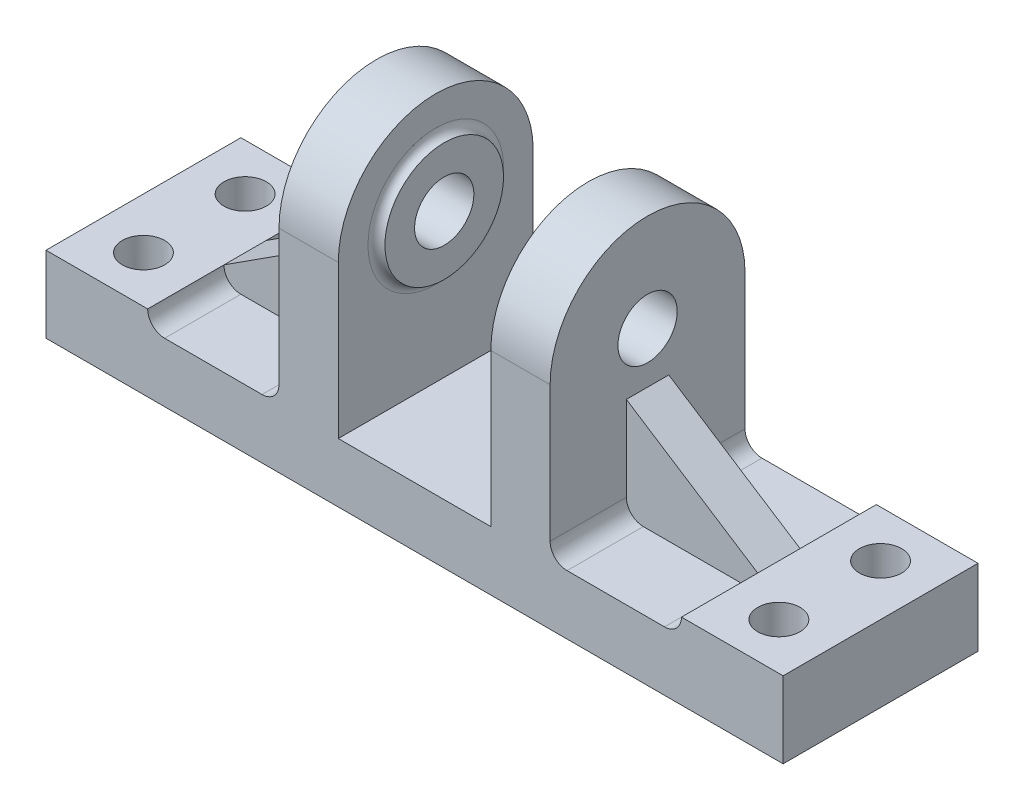
ISO-10303-21;
HEADER;
FILE_DESCRIPTION(('STEP AP214'),'2;1');
FILE_NAME('part.step','',(''),(''),'','','');
FILE_SCHEMA(('AUTOMOTIVE_DESIGN { 1 0 10303 214 1 1 1 1 }'));
ENDSEC;
DATA;
#1=APPLICATION_CONTEXT('core data for automotive mechanical design processes');
#2=APPLICATION_PROTOCOL_DEFINITION('international standard','automotive_design',2000,#1);
#3=PRODUCT_CONTEXT('',#1,'mechanical');
#4=PRODUCT('Part','Part','',(#3));
#5=PRODUCT_RELATED_PRODUCT_CATEGORY('part','',(#4));
#6=PRODUCT_DEFINITION_FORMATION('','',#4);
#7=PRODUCT_DEFINITION_CONTEXT('part definition',#1,'design');
#8=PRODUCT_DEFINITION('design','',#6,#7);
#9=PRODUCT_DEFINITION_SHAPE('','',#8);
#10=(LENGTH_UNIT() NAMED_UNIT(*) SI_UNIT(.MILLI.,.METRE.));
#11=(NAMED_UNIT(*) PLANE_ANGLE_UNIT() SI_UNIT($,.RADIAN.));
#12=(NAMED_UNIT(*) SI_UNIT($,.STERADIAN.) SOLID_ANGLE_UNIT());
#13=UNCERTAINTY_MEASURE_WITH_UNIT(LENGTH_MEASURE(1.E-05),#10,'distance_accuracy_value','');
#14=(GEOMETRIC_REPRESENTATION_CONTEXT(3) GLOBAL_UNCERTAINTY_ASSIGNED_CONTEXT((#13)) GLOBAL_UNIT_ASSIGNED_CONTEXT((#10,
#11,#12)) REPRESENTATION_CONTEXT('',''));
#15=CARTESIAN_POINT('',(0.,0.,0.));
#16=DIRECTION('',(0.,0.,1.));
#17=DIRECTION('',(1.,0.,0.));
#18=AXIS2_PLACEMENT_3D('',#15,#16,#17);
#19=CARTESIAN_POINT('',(63.,5.00000000000001,23.));
#20=DIRECTION('',(0.,-1.,0.));
#21=DIRECTION('',(1.,0.,0.));
#22=AXIS2_PLACEMENT_3D('',#19,#20,#21);
#23=PLANE('',#22);
#24=DIRECTION('',(-1.,0.,0.));
#25=VECTOR('',#24,1.);
#26=CARTESIAN_POINT('',(63.,5.00000000000001,-5.));
#27=LINE('',#26,#25);
#28=CARTESIAN_POINT('',(-36.,5.,-5.));
#29=VERTEX_POINT('',#28);
#30=CARTESIAN_POINT('',(-59.,5.,-5.));
#31=VERTEX_POINT('',#30);
#32=EDGE_CURVE('E245',#29,#31,#27,.T.);
#33=ORIENTED_EDGE('',*,*,#32,.F.);
#34=DIRECTION('',(0.,0.,-1.));
#35=VECTOR('',#34,1.);
#36=CARTESIAN_POINT('',(-36.,5.,23.));
#37=LINE('',#36,#35);
#38=CARTESIAN_POINT('',(-36.,5.,-23.));
#39=VERTEX_POINT('',#38);
#40=EDGE_CURVE('E227',#29,#39,#37,.T.);
#41=ORIENTED_EDGE('',*,*,#40,.T.);
#42=DIRECTION('',(-1.,0.,0.));
#43=VECTOR('',#42,1.);
#44=CARTESIAN_POINT('',(63.,5.00000000000001,-23.));
#45=LINE('',#44,#43);
#46=CARTESIAN_POINT('',(-59.,5.,-23.));
#47=VERTEX_POINT('',#46);
#48=EDGE_CURVE('E328',#39,#47,#45,.T.);
#49=ORIENTED_EDGE('',*,*,#48,.T.);
#50=DIRECTION('',(0.,0.,-1.));
#51=VECTOR('',#50,1.);
#52=CARTESIAN_POINT('',(-59.,5.,23.));
#53=LINE('',#52,#51);
#54=EDGE_CURVE('E242',#47,#31,#53,.F.);
#55=ORIENTED_EDGE('',*,*,#54,.T.);
#56=EDGE_LOOP('',(#33,#41,#49,#55));
#57=FACE_BOUND('',#56,.T.);
#58=ADVANCED_FACE('F41',(#57),#23,.F.);
#59=CARTESIAN_POINT('',(-59.,9.,23.));
#60=DIRECTION('',(0.,0.,1.));
#61=DIRECTION('',(1.,0.,0.));
#62=AXIS2_PLACEMENT_3D('',#59,#60,#61);
#63=CYLINDRICAL_SURFACE('',#62,4.);
#64=CARTESIAN_POINT('',(-59.,9.,-5.));
#65=DIRECTION('',(0.,0.,1.));
#66=DIRECTION('',(1.,0.,0.));
#67=AXIS2_PLACEMENT_3D('',#64,#65,#66);
#68=CIRCLE('',#67,4.);
#69=CARTESIAN_POINT('',(-63.,8.99999999999999,-5.));
#70=VERTEX_POINT('',#69);
#71=EDGE_CURVE('E250',#31,#70,#68,.F.);
#72=ORIENTED_EDGE('',*,*,#71,.F.);
#73=ORIENTED_EDGE('',*,*,#54,.F.);
#74=CARTESIAN_POINT('',(-59.,9.,-23.));
#75=DIRECTION('',(0.,0.,1.));
#76=DIRECTION('',(1.,0.,0.));
#77=AXIS2_PLACEMENT_3D('',#74,#75,#76);
#78=CIRCLE('',#77,4.);
#79=CARTESIAN_POINT('',(-63.,8.99999999999999,-23.));
#80=VERTEX_POINT('',#79);
#81=EDGE_CURVE('E286',#80,#47,#78,.T.);
#82=ORIENTED_EDGE('',*,*,#81,.F.);
#83=DIRECTION('',(0.,0.,-1.));
#84=VECTOR('',#83,1.);
#85=CARTESIAN_POINT('',(-63.,8.99999999999999,23.));
#86=LINE('',#85,#84);
#87=EDGE_CURVE('E57',#70,#80,#86,.T.);
#88=ORIENTED_EDGE('',*,*,#87,.F.);
#89=EDGE_LOOP('',(#72,#73,#82,#88));
#90=FACE_BOUND('',#89,.T.);
#91=ADVANCED_FACE('F595',(#90),#63,.F.);
#92=CARTESIAN_POINT('',(-36.,9.,23.));
#93=DIRECTION('',(0.,0.,-1.));
#94=DIRECTION('',(-1.,0.,0.));
#95=AXIS2_PLACEMENT_3D('',#92,#93,#94);
#96=CYLINDRICAL_SURFACE('',#95,4.);
#97=CARTESIAN_POINT('',(-36.,9.,-5.));
#98=DIRECTION('',(0.,0.,1.));
#99=DIRECTION('',(1.,0.,0.));
#100=AXIS2_PLACEMENT_3D('',#97,#98,#99);
#101=CIRCLE('',#100,4.);
#102=CARTESIAN_POINT('',(-32.,9.,-5.));
#103=VERTEX_POINT('',#102);
#104=EDGE_CURVE('E235',#103,#29,#101,.F.);
#105=ORIENTED_EDGE('',*,*,#104,.F.);
#106=DIRECTION('',(0.,0.,-1.));
#107=VECTOR('',#106,1.);
#108=CARTESIAN_POINT('',(-32.,9.,0.));
#109=LINE('',#108,#107);
#110=CARTESIAN_POINT('',(-32.,9.,-23.));
#111=VERTEX_POINT('',#110);
#112=EDGE_CURVE('E259',#111,#103,#109,.F.);
#113=ORIENTED_EDGE('',*,*,#112,.F.);
#114=CARTESIAN_POINT('',(-36.,9.,-23.));
#115=DIRECTION('',(0.,0.,1.));
#116=DIRECTION('',(1.,0.,0.));
#117=AXIS2_PLACEMENT_3D('',#114,#115,#116);
#118=CIRCLE('',#117,4.);
#119=EDGE_CURVE('E234',#39,#111,#118,.T.);
#120=ORIENTED_EDGE('',*,*,#119,.F.);
#121=ORIENTED_EDGE('',*,*,#40,.F.);
#122=EDGE_LOOP('',(#105,#113,#120,#121));
#123=FACE_BOUND('',#122,.T.);
#124=ADVANCED_FACE('F230',(#123),#96,.F.);
#125=CARTESIAN_POINT('',(-18.,0.,0.));
#126=DIRECTION('',(-1.,0.,0.));
#127=DIRECTION('',(0.,0.,-1.));
#128=AXIS2_PLACEMENT_3D('',#125,#126,#127);
#129=PLANE('',#128);
#130=CARTESIAN_POINT('',(-18.,41.,0.));
#131=DIRECTION('',(-1.,0.,0.));
#132=DIRECTION('',(0.,0.,1.));
#133=AXIS2_PLACEMENT_3D('',#130,#131,#132);
#134=CIRCLE('',#133,16.);
#135=CARTESIAN_POINT('',(-18.,41.,16.));
#136=VERTEX_POINT('',#135);
#137=EDGE_CURVE('E238',#136,#136,#134,.T.);
#138=ORIENTED_EDGE('',*,*,#137,.T.);
#139=EDGE_LOOP('',(#138));
#140=FACE_BOUND('',#139,.T.);
#141=DIRECTION('',(0.,0.,-1.));
#142=VECTOR('',#141,1.);
#143=CARTESIAN_POINT('',(-18.,5.00000000000002,0.));
#144=LINE('',#143,#142);
#145=CARTESIAN_POINT('',(-18.,5.,23.));
#146=VERTEX_POINT('',#145);
#147=CARTESIAN_POINT('',(-18.,5.,-23.));
#148=VERTEX_POINT('',#147);
#149=EDGE_CURVE('E453',#146,#148,#144,.T.);
#150=ORIENTED_EDGE('',*,*,#149,.T.);
#151=DIRECTION('',(0.,-1.,0.));
#152=VECTOR('',#151,1.);
#153=CARTESIAN_POINT('',(-18.,0.,-23.));
#154=LINE('',#153,#152);
#155=CARTESIAN_POINT('',(-18.,41.,-23.));
#156=VERTEX_POINT('',#155);
#157=EDGE_CURVE('E459',#156,#148,#154,.T.);
#158=ORIENTED_EDGE('',*,*,#157,.F.);
#159=CARTESIAN_POINT('',(-18.,41.,0.));
#160=DIRECTION('',(1.,0.,0.));
#161=DIRECTION('',(0.,0.,-1.));
#162=AXIS2_PLACEMENT_3D('',#159,#160,#161);
#163=CIRCLE('',#162,23.);
#164=CARTESIAN_POINT('',(-18.,41.,23.));
#165=VERTEX_POINT('',#164);
#166=EDGE_CURVE('E445',#165,#156,#163,.F.);
#167=ORIENTED_EDGE('',*,*,#166,.F.);
#168=DIRECTION('',(0.,-1.,0.));
#169=VECTOR('',#168,1.);
#170=CARTESIAN_POINT('',(-18.,0.,23.));
#171=LINE('',#170,#169);
#172=EDGE_CURVE('E440',#165,#146,#171,.T.);
#173=ORIENTED_EDGE('',*,*,#172,.T.);
#174=EDGE_LOOP('',(#150,#158,#167,#173));
#175=FACE_BOUND('',#174,.T.);
#176=ADVANCED_FACE('F515',(#140,#175),#129,.F.);
#177=DIRECTION('',(0.,0.,-1.));
#178=VECTOR('',#177,1.);
#179=CARTESIAN_POINT('',(18.,5.00000000000002,0.));
#180=LINE('',#179,#178);
#181=CARTESIAN_POINT('',(18.,5.,23.));
#182=VERTEX_POINT('',#181);
#183=CARTESIAN_POINT('',(18.,5.00000000000002,-23.));
#184=VERTEX_POINT('',#183);
#185=EDGE_CURVE('E399',#182,#184,#180,.T.);
#186=ORIENTED_EDGE('',*,*,#185,.T.);
#187=EDGE_CURVE('E323',#184,#148,#45,.T.);
#188=ORIENTED_EDGE('',*,*,#187,.T.);
#189=ORIENTED_EDGE('',*,*,#149,.F.);
#190=DIRECTION('',(-1.,0.,0.));
#191=VECTOR('',#190,1.);
#192=CARTESIAN_POINT('',(63.,5.00000000000001,23.));
#193=LINE('',#192,#191);
#194=EDGE_CURVE('E341',#182,#146,#193,.T.);
#195=ORIENTED_EDGE('',*,*,#194,.F.);
#196=EDGE_LOOP('',(#186,#188,#189,#195));
#197=FACE_BOUND('',#196,.T.);
#198=ADVANCED_FACE('F525',(#197),#23,.F.);
#199=DIRECTION('',(-1.,0.,0.));
#200=VECTOR('',#199,1.);
#201=CARTESIAN_POINT('',(63.,5.00000000000001,-5.));
#202=LINE('',#201,#200);
#203=CARTESIAN_POINT('',(59.,5.00000000000001,-5.));
#204=VERTEX_POINT('',#203);
#205=CARTESIAN_POINT('',(36.,5.00000000000001,-5.));
#206=VERTEX_POINT('',#205);
#207=EDGE_CURVE('E422',#204,#206,#202,.T.);
#208=ORIENTED_EDGE('',*,*,#207,.F.);
#209=DIRECTION('',(0.,0.,-1.));
#210=VECTOR('',#209,1.);
#211=CARTESIAN_POINT('',(59.,5.00000000000001,-23.));
#212=LINE('',#211,#210);
#213=CARTESIAN_POINT('',(59.,5.00000000000001,-23.));
#214=VERTEX_POINT('',#213);
#215=EDGE_CURVE('E297',#204,#214,#212,.T.);
#216=ORIENTED_EDGE('',*,*,#215,.T.);
#217=CARTESIAN_POINT('',(36.,5.00000000000001,-23.));
#218=VERTEX_POINT('',#217);
#219=EDGE_CURVE('E325',#214,#218,#45,.T.);
#220=ORIENTED_EDGE('',*,*,#219,.T.);
#221=DIRECTION('',(0.,0.,-1.));
#222=VECTOR('',#221,1.);
#223=CARTESIAN_POINT('',(36.,5.00000000000001,23.));
#224=LINE('',#223,#222);
#225=EDGE_CURVE('E277',#218,#206,#224,.F.);
#226=ORIENTED_EDGE('',*,*,#225,.T.);
#227=EDGE_LOOP('',(#208,#216,#220,#226));
#228=FACE_BOUND('',#227,.T.);
#229=ADVANCED_FACE('F542',(#228),#23,.F.);
#230=CARTESIAN_POINT('',(59.,9.00000000000001,23.));
#231=DIRECTION('',(0.,0.,1.));
#232=DIRECTION('',(1.,0.,0.));
#233=AXIS2_PLACEMENT_3D('',#230,#231,#232);
#234=CYLINDRICAL_SURFACE('',#233,4.);
#235=CARTESIAN_POINT('',(59.,9.00000000000001,-5.));
#236=DIRECTION('',(0.,0.,1.));
#237=DIRECTION('',(1.,0.,0.));
#238=AXIS2_PLACEMENT_3D('',#235,#236,#237);
#239=CIRCLE('',#238,4.);
#240=CARTESIAN_POINT('',(63.,9.00000000000001,-5.));
#241=VERTEX_POINT('',#240);
#242=EDGE_CURVE('E416',#241,#204,#239,.F.);
#243=ORIENTED_EDGE('',*,*,#242,.F.);
#244=DIRECTION('',(0.,0.,-1.));
#245=VECTOR('',#244,1.);
#246=CARTESIAN_POINT('',(63.,9.00000000000001,23.));
#247=LINE('',#246,#245);
#248=CARTESIAN_POINT('',(63.,9.00000000000001,-23.));
#249=VERTEX_POINT('',#248);
#250=EDGE_CURVE('E315',#241,#249,#247,.T.);
#251=ORIENTED_EDGE('',*,*,#250,.T.);
#252=CARTESIAN_POINT('',(59.,9.00000000000001,-23.));
#253=DIRECTION('',(0.,0.,1.));
#254=DIRECTION('',(1.,0.,0.));
#255=AXIS2_PLACEMENT_3D('',#252,#253,#254);
#256=CIRCLE('',#255,4.);
#257=EDGE_CURVE('E295',#214,#249,#256,.T.);
#258=ORIENTED_EDGE('',*,*,#257,.F.);
#259=ORIENTED_EDGE('',*,*,#215,.F.);
#260=EDGE_LOOP('',(#243,#251,#258,#259));
#261=FACE_BOUND('',#260,.T.);
#262=ADVANCED_FACE('F548',(#261),#234,.F.);
#263=CARTESIAN_POINT('',(36.,9.00000000000001,0.));
#264=DIRECTION('',(0.,0.,-1.));
#265=DIRECTION('',(-1.,0.,0.));
#266=AXIS2_PLACEMENT_3D('',#263,#264,#265);
#267=CYLINDRICAL_SURFACE('',#266,4.);
#268=CARTESIAN_POINT('',(36.,9.00000000000001,-5.));
#269=DIRECTION('',(0.,0.,1.));
#270=DIRECTION('',(1.,0.,0.));
#271=AXIS2_PLACEMENT_3D('',#268,#269,#270);
#272=CIRCLE('',#271,4.);
#273=CARTESIAN_POINT('',(32.,9.00000000000001,-5.));
#274=VERTEX_POINT('',#273);
#275=EDGE_CURVE('E266',#206,#274,#272,.F.);
#276=ORIENTED_EDGE('',*,*,#275,.F.);
#277=ORIENTED_EDGE('',*,*,#225,.F.);
#278=CARTESIAN_POINT('',(36.,9.00000000000001,-23.));
#279=DIRECTION('',(0.,0.,1.));
#280=DIRECTION('',(1.,0.,0.));
#281=AXIS2_PLACEMENT_3D('',#278,#279,#280);
#282=CIRCLE('',#281,4.);
#283=CARTESIAN_POINT('',(32.,9.00000000000001,-23.));
#284=VERTEX_POINT('',#283);
#285=EDGE_CURVE('E274',#284,#218,#282,.T.);
#286=ORIENTED_EDGE('',*,*,#285,.F.);
#287=DIRECTION('',(0.,0.,-1.));
#288=VECTOR('',#287,1.);
#289=CARTESIAN_POINT('',(32.,9.00000000000001,0.));
#290=LINE('',#289,#288);
#291=EDGE_CURVE('E282',#274,#284,#290,.T.);
#292=ORIENTED_EDGE('',*,*,#291,.F.);
#293=EDGE_LOOP('',(#276,#277,#286,#292));
#294=FACE_BOUND('',#293,.T.);
#295=ADVANCED_FACE('F543',(#294),#267,.F.);
#296=CARTESIAN_POINT('',(-36.,5.,23.));
#297=VERTEX_POINT('',#296);
#298=CARTESIAN_POINT('',(-36.,5.,5.));
#299=VERTEX_POINT('',#298);
#300=EDGE_CURVE('E240',#297,#299,#37,.T.);
#301=ORIENTED_EDGE('',*,*,#300,.T.);
#302=DIRECTION('',(-1.,0.,0.));
#303=VECTOR('',#302,1.);
#304=CARTESIAN_POINT('',(63.,5.00000000000001,5.));
#305=LINE('',#304,#303);
#306=CARTESIAN_POINT('',(-59.,5.,5.));
#307=VERTEX_POINT('',#306);
#308=EDGE_CURVE('E468',#299,#307,#305,.T.);
#309=ORIENTED_EDGE('',*,*,#308,.T.);
#310=CARTESIAN_POINT('',(-59.,5.,23.));
#311=VERTEX_POINT('',#310);
#312=EDGE_CURVE('E305',#307,#311,#53,.F.);
#313=ORIENTED_EDGE('',*,*,#312,.T.);
#314=EDGE_CURVE('E343',#297,#311,#193,.T.);
#315=ORIENTED_EDGE('',*,*,#314,.F.);
#316=EDGE_LOOP('',(#301,#309,#313,#315));
#317=FACE_BOUND('',#316,.T.);
#318=ADVANCED_FACE('F502',(#317),#23,.F.);
#319=CARTESIAN_POINT('',(-87.,-9.,23.));
#320=DIRECTION('',(1.,0.,0.));
#321=DIRECTION('',(0.,0.,-1.));
#322=AXIS2_PLACEMENT_3D('',#319,#320,#321);
#323=PLANE('',#322);
#324=DIRECTION('',(0.,-1.,0.));
#325=VECTOR('',#324,1.);
#326=CARTESIAN_POINT('',(-87.,-9.,-23.));
#327=LINE('',#326,#325);
#328=CARTESIAN_POINT('',(-87.,9.,-23.));
#329=VERTEX_POINT('',#328);
#330=CARTESIAN_POINT('',(-87.,-9.,-23.));
#331=VERTEX_POINT('',#330);
#332=EDGE_CURVE('E337',#329,#331,#327,.T.);
#333=ORIENTED_EDGE('',*,*,#332,.T.);
#334=DIRECTION('',(0.,0.,-1.));
#335=VECTOR('',#334,1.);
#336=CARTESIAN_POINT('',(-87.,-9.,23.));
#337=LINE('',#336,#335);
#338=CARTESIAN_POINT('',(-87.,-9.,23.));
#339=VERTEX_POINT('',#338);
#340=EDGE_CURVE('E303',#339,#331,#337,.T.);
#341=ORIENTED_EDGE('',*,*,#340,.F.);
#342=DIRECTION('',(0.,-1.,0.));
#343=VECTOR('',#342,1.);
#344=CARTESIAN_POINT('',(-87.,-9.,23.));
#345=LINE('',#344,#343);
#346=CARTESIAN_POINT('',(-87.,9.,23.));
#347=VERTEX_POINT('',#346);
#348=EDGE_CURVE('E322',#347,#339,#345,.T.);
#349=ORIENTED_EDGE('',*,*,#348,.F.);
#350=DIRECTION('',(0.,0.,-1.));
#351=VECTOR('',#350,1.);
#352=CARTESIAN_POINT('',(-87.,9.,23.));
#353=LINE('',#352,#351);
#354=EDGE_CURVE('E314',#347,#329,#353,.T.);
#355=ORIENTED_EDGE('',*,*,#354,.T.);
#356=EDGE_LOOP('',(#333,#341,#349,#355));
#357=FACE_BOUND('',#356,.T.);
#358=ADVANCED_FACE('F614',(#357),#323,.F.);
#359=CARTESIAN_POINT('',(87.,-8.99999999999998,23.));
#360=DIRECTION('',(0.,1.,0.));
#361=DIRECTION('',(-1.,0.,0.));
#362=AXIS2_PLACEMENT_3D('',#359,#360,#361);
#363=PLANE('',#362);
#364=CARTESIAN_POINT('',(75.,-8.99999999999998,12.));
#365=DIRECTION('',(0.,1.,0.));
#366=DIRECTION('',(-1.,0.,0.));
#367=AXIS2_PLACEMENT_3D('',#364,#365,#366);
#368=CIRCLE('',#367,5.);
#369=CARTESIAN_POINT('',(70.,-8.99999999999998,12.));
#370=VERTEX_POINT('',#369);
#371=EDGE_CURVE('E358',#370,#370,#368,.T.);
#372=ORIENTED_EDGE('',*,*,#371,.T.);
#373=EDGE_LOOP('',(#372));
#374=FACE_BOUND('',#373,.T.);
#375=CARTESIAN_POINT('',(-75.,-9.,12.));
#376=DIRECTION('',(0.,1.,0.));
#377=DIRECTION('',(-1.,0.,0.));
#378=AXIS2_PLACEMENT_3D('',#375,#376,#377);
#379=CIRCLE('',#378,5.);
#380=CARTESIAN_POINT('',(-80.,-9.,12.));
#381=VERTEX_POINT('',#380);
#382=EDGE_CURVE('E360',#381,#381,#379,.T.);
#383=ORIENTED_EDGE('',*,*,#382,.T.);
#384=EDGE_LOOP('',(#383));
#385=FACE_BOUND('',#384,.T.);
#386=ORIENTED_EDGE('',*,*,#340,.T.);
#387=DIRECTION('',(1.,0.,0.));
#388=VECTOR('',#387,1.);
#389=CARTESIAN_POINT('',(87.,-8.99999999999998,-23.));
#390=LINE('',#389,#388);
#391=CARTESIAN_POINT('',(87.,-8.99999999999998,-23.));
#392=VERTEX_POINT('',#391);
#393=EDGE_CURVE('E334',#331,#392,#390,.T.);
#394=ORIENTED_EDGE('',*,*,#393,.T.);
#395=DIRECTION('',(0.,0.,-1.));
#396=VECTOR('',#395,1.);
#397=CARTESIAN_POINT('',(87.,-8.99999999999998,23.));
#398=LINE('',#397,#396);
#399=CARTESIAN_POINT('',(87.,-8.99999999999998,23.));
#400=VERTEX_POINT('',#399);
#401=EDGE_CURVE('E304',#400,#392,#398,.T.);
#402=ORIENTED_EDGE('',*,*,#401,.F.);
#403=DIRECTION('',(1.,0.,0.));
#404=VECTOR('',#403,1.);
#405=CARTESIAN_POINT('',(87.,-8.99999999999998,23.));
#406=LINE('',#405,#404);
#407=EDGE_CURVE('E346',#339,#400,#406,.T.);
#408=ORIENTED_EDGE('',*,*,#407,.F.);
#409=EDGE_LOOP('',(#386,#394,#402,#408));
#410=FACE_BOUND('',#409,.T.);
#411=CARTESIAN_POINT('',(75.,-8.99999999999998,-12.));
#412=DIRECTION('',(0.,1.,0.));
#413=DIRECTION('',(-1.,0.,0.));
#414=AXIS2_PLACEMENT_3D('',#411,#412,#413);
#415=CIRCLE('',#414,5.);
#416=CARTESIAN_POINT('',(70.,-8.99999999999998,-12.));
#417=VERTEX_POINT('',#416);
#418=EDGE_CURVE('E339',#417,#417,#415,.T.);
#419=ORIENTED_EDGE('',*,*,#418,.T.);
#420=EDGE_LOOP('',(#419));
#421=FACE_BOUND('',#420,.T.);
#422=CARTESIAN_POINT('',(-75.,-9.,-12.));
#423=DIRECTION('',(0.,1.,0.));
#424=DIRECTION('',(-1.,0.,0.));
#425=AXIS2_PLACEMENT_3D('',#422,#423,#424);
#426=CIRCLE('',#425,5.);
#427=CARTESIAN_POINT('',(-80.,-9.,-12.));
#428=VERTEX_POINT('',#427);
#429=EDGE_CURVE('E365',#428,#428,#426,.T.);
#430=ORIENTED_EDGE('',*,*,#429,.T.);
#431=EDGE_LOOP('',(#430));
#432=FACE_BOUND('',#431,.T.);
#433=ADVANCED_FACE('F617',(#374,#385,#410,#421,#432),#363,.F.);
#434=CARTESIAN_POINT('',(87.,-8.99999999999998,23.));
#435=DIRECTION('',(-1.,0.,0.));
#436=DIRECTION('',(0.,0.,1.));
#437=AXIS2_PLACEMENT_3D('',#434,#435,#436);
#438=PLANE('',#437);
#439=ORIENTED_EDGE('',*,*,#401,.T.);
#440=DIRECTION('',(0.,1.,0.));
#441=VECTOR('',#440,1.);
#442=CARTESIAN_POINT('',(87.,-8.99999999999998,-23.));
#443=LINE('',#442,#441);
#444=CARTESIAN_POINT('',(87.,9.00000000000002,-23.));
#445=VERTEX_POINT('',#444);
#446=EDGE_CURVE('E326',#392,#445,#443,.T.);
#447=ORIENTED_EDGE('',*,*,#446,.T.);
#448=DIRECTION('',(0.,0.,-1.));
#449=VECTOR('',#448,1.);
#450=CARTESIAN_POINT('',(87.,9.00000000000002,23.));
#451=LINE('',#450,#449);
#452=CARTESIAN_POINT('',(87.,9.00000000000002,23.));
#453=VERTEX_POINT('',#452);
#454=EDGE_CURVE('E310',#453,#445,#451,.T.);
#455=ORIENTED_EDGE('',*,*,#454,.F.);
#456=DIRECTION('',(0.,1.,0.));
#457=VECTOR('',#456,1.);
#458=CARTESIAN_POINT('',(87.,-8.99999999999998,23.));
#459=LINE('',#458,#457);
#460=EDGE_CURVE('E347',#400,#453,#459,.T.);
#461=ORIENTED_EDGE('',*,*,#460,.F.);
#462=EDGE_LOOP('',(#439,#447,#455,#461));
#463=FACE_BOUND('',#462,.T.);
#464=ADVANCED_FACE('F606',(#463),#438,.F.);
#465=CARTESIAN_POINT('',(87.,9.00000000000002,23.));
#466=DIRECTION('',(0.,-1.,0.));
#467=DIRECTION('',(1.,0.,0.));
#468=AXIS2_PLACEMENT_3D('',#465,#466,#467);
#469=PLANE('',#468);
#470=CARTESIAN_POINT('',(75.,8.99999999999998,12.));
#471=DIRECTION('',(0.,1.,0.));
#472=DIRECTION('',(-1.,0.,0.));
#473=AXIS2_PLACEMENT_3D('',#470,#471,#472);
#474=CIRCLE('',#473,5.);
#475=CARTESIAN_POINT('',(70.,8.99999999999998,12.));
#476=VERTEX_POINT('',#475);
#477=EDGE_CURVE('E375',#476,#476,#474,.T.);
#478=ORIENTED_EDGE('',*,*,#477,.F.);
#479=EDGE_LOOP('',(#478));
#480=FACE_BOUND('',#479,.T.);
#481=ORIENTED_EDGE('',*,*,#454,.T.);
#482=DIRECTION('',(-1.,0.,0.));
#483=VECTOR('',#482,1.);
#484=CARTESIAN_POINT('',(87.,9.00000000000002,-23.));
#485=LINE('',#484,#483);
#486=EDGE_CURVE('E329',#445,#249,#485,.T.);
#487=ORIENTED_EDGE('',*,*,#486,.T.);
#488=ORIENTED_EDGE('',*,*,#250,.F.);
#489=DIRECTION('',(0.,0.,1.));
#490=VECTOR('',#489,1.);
#491=CARTESIAN_POINT('',(63.,9.00000000000001,23.));
#492=LINE('',#491,#490);
#493=CARTESIAN_POINT('',(63.,9.00000000000001,5.));
#494=VERTEX_POINT('',#493);
#495=EDGE_CURVE('E408',#241,#494,#492,.T.);
#496=ORIENTED_EDGE('',*,*,#495,.T.);
#497=CARTESIAN_POINT('',(63.,9.00000000000001,23.));
#498=VERTEX_POINT('',#497);
#499=EDGE_CURVE('E307',#498,#494,#247,.T.);
#500=ORIENTED_EDGE('',*,*,#499,.F.);
#501=DIRECTION('',(-1.,0.,0.));
#502=VECTOR('',#501,1.);
#503=CARTESIAN_POINT('',(87.,9.00000000000002,23.));
#504=LINE('',#503,#502);
#505=EDGE_CURVE('E348',#453,#498,#504,.T.);
#506=ORIENTED_EDGE('',*,*,#505,.F.);
#507=EDGE_LOOP('',(#481,#487,#488,#496,#500,#506));
#508=FACE_BOUND('',#507,.T.);
#509=CARTESIAN_POINT('',(75.,8.99999999999998,-12.));
#510=DIRECTION('',(0.,1.,0.));
#511=DIRECTION('',(1.,0.,0.));
#512=AXIS2_PLACEMENT_3D('',#509,#510,#511);
#513=CIRCLE('',#512,5.);
#514=CARTESIAN_POINT('',(80.,8.99999999999998,-12.));
#515=VERTEX_POINT('',#514);
#516=EDGE_CURVE('E367',#515,#515,#513,.T.);
#517=ORIENTED_EDGE('',*,*,#516,.F.);
#518=EDGE_LOOP('',(#517));
#519=FACE_BOUND('',#518,.T.);
#520=ADVANCED_FACE('F555',(#480,#508,#519),#469,.F.);
#521=CARTESIAN_POINT('',(59.,5.00000000000001,23.));
#522=VERTEX_POINT('',#521);
#523=CARTESIAN_POINT('',(59.,5.00000000000001,5.));
#524=VERTEX_POINT('',#523);
#525=EDGE_CURVE('E300',#522,#524,#212,.T.);
#526=ORIENTED_EDGE('',*,*,#525,.T.);
#527=DIRECTION('',(-1.,0.,0.));
#528=VECTOR('',#527,1.);
#529=CARTESIAN_POINT('',(63.,5.00000000000001,5.));
#530=LINE('',#529,#528);
#531=CARTESIAN_POINT('',(36.,5.00000000000001,5.));
#532=VERTEX_POINT('',#531);
#533=EDGE_CURVE('E415',#524,#532,#530,.T.);
#534=ORIENTED_EDGE('',*,*,#533,.T.);
#535=CARTESIAN_POINT('',(36.,5.00000000000001,23.));
#536=VERTEX_POINT('',#535);
#537=EDGE_CURVE('E276',#532,#536,#224,.F.);
#538=ORIENTED_EDGE('',*,*,#537,.T.);
#539=EDGE_CURVE('E342',#522,#536,#193,.T.);
#540=ORIENTED_EDGE('',*,*,#539,.F.);
#541=EDGE_LOOP('',(#526,#534,#538,#540));
#542=FACE_BOUND('',#541,.T.);
#543=ADVANCED_FACE('F575',(#542),#23,.F.);
#544=CARTESIAN_POINT('',(-63.,8.99999999999999,23.));
#545=DIRECTION('',(0.,-1.,0.));
#546=DIRECTION('',(1.,0.,0.));
#547=AXIS2_PLACEMENT_3D('',#544,#545,#546);
#548=PLANE('',#547);
#549=CARTESIAN_POINT('',(-75.,8.99999999999999,12.));
#550=DIRECTION('',(0.,1.,0.));
#551=DIRECTION('',(1.,0.,0.));
#552=AXIS2_PLACEMENT_3D('',#549,#550,#551);
#553=CIRCLE('',#552,5.);
#554=CARTESIAN_POINT('',(-70.,8.99999999999999,12.));
#555=VERTEX_POINT('',#554);
#556=EDGE_CURVE('E368',#555,#555,#553,.T.);
#557=ORIENTED_EDGE('',*,*,#556,.F.);
#558=EDGE_LOOP('',(#557));
#559=FACE_BOUND('',#558,.T.);
#560=CARTESIAN_POINT('',(-63.,8.99999999999999,23.));
#561=VERTEX_POINT('',#560);
#562=CARTESIAN_POINT('',(-63.,8.99999999999999,5.));
#563=VERTEX_POINT('',#562);
#564=EDGE_CURVE('E312',#561,#563,#86,.T.);
#565=ORIENTED_EDGE('',*,*,#564,.T.);
#566=DIRECTION('',(0.,0.,1.));
#567=VECTOR('',#566,1.);
#568=CARTESIAN_POINT('',(-63.,8.99999999999999,23.));
#569=LINE('',#568,#567);
#570=EDGE_CURVE('E470',#563,#70,#569,.F.);
#571=ORIENTED_EDGE('',*,*,#570,.T.);
#572=ORIENTED_EDGE('',*,*,#87,.T.);
#573=DIRECTION('',(-1.,0.,0.));
#574=VECTOR('',#573,1.);
#575=CARTESIAN_POINT('',(-63.,8.99999999999999,-23.));
#576=LINE('',#575,#574);
#577=EDGE_CURVE('E319',#80,#329,#576,.T.);
#578=ORIENTED_EDGE('',*,*,#577,.T.);
#579=ORIENTED_EDGE('',*,*,#354,.F.);
#580=DIRECTION('',(-1.,0.,0.));
#581=VECTOR('',#580,1.);
#582=CARTESIAN_POINT('',(-63.,8.99999999999999,23.));
#583=LINE('',#582,#581);
#584=EDGE_CURVE('E320',#561,#347,#583,.T.);
#585=ORIENTED_EDGE('',*,*,#584,.F.);
#586=EDGE_LOOP('',(#565,#571,#572,#578,#579,#585));
#587=FACE_BOUND('',#586,.T.);
#588=CARTESIAN_POINT('',(-75.,8.99999999999999,-12.));
#589=DIRECTION('',(0.,1.,0.));
#590=DIRECTION('',(-1.,0.,0.));
#591=AXIS2_PLACEMENT_3D('',#588,#589,#590);
#592=CIRCLE('',#591,5.);
#593=CARTESIAN_POINT('',(-80.,8.99999999999999,-12.));
#594=VERTEX_POINT('',#593);
#595=EDGE_CURVE('E362',#594,#594,#592,.T.);
#596=ORIENTED_EDGE('',*,*,#595,.F.);
#597=EDGE_LOOP('',(#596));
#598=FACE_BOUND('',#597,.T.);
#599=ADVANCED_FACE('F601',(#559,#587,#598),#548,.F.);
#600=CARTESIAN_POINT('',(0.,0.,23.));
#601=DIRECTION('',(0.,0.,1.));
#602=DIRECTION('',(1.,0.,0.));
#603=AXIS2_PLACEMENT_3D('',#600,#601,#602);
#604=PLANE('',#603);
#605=ORIENTED_EDGE('',*,*,#348,.T.);
#606=ORIENTED_EDGE('',*,*,#407,.T.);
#607=ORIENTED_EDGE('',*,*,#460,.T.);
#608=ORIENTED_EDGE('',*,*,#505,.T.);
#609=CARTESIAN_POINT('',(59.,9.00000000000001,23.));
#610=DIRECTION('',(0.,0.,1.));
#611=DIRECTION('',(1.,0.,0.));
#612=AXIS2_PLACEMENT_3D('',#609,#610,#611);
#613=CIRCLE('',#612,4.);
#614=EDGE_CURVE('E292',#498,#522,#613,.F.);
#615=ORIENTED_EDGE('',*,*,#614,.T.);
#616=ORIENTED_EDGE('',*,*,#539,.T.);
#617=CARTESIAN_POINT('',(36.,9.00000000000001,23.));
#618=DIRECTION('',(0.,0.,1.));
#619=DIRECTION('',(1.,0.,0.));
#620=AXIS2_PLACEMENT_3D('',#617,#618,#619);
#621=CIRCLE('',#620,4.);
#622=CARTESIAN_POINT('',(32.,9.00000000000001,23.));
#623=VERTEX_POINT('',#622);
#624=EDGE_CURVE('E275',#536,#623,#621,.F.);
#625=ORIENTED_EDGE('',*,*,#624,.T.);
#626=DIRECTION('',(0.,-1.,0.));
#627=VECTOR('',#626,1.);
#628=CARTESIAN_POINT('',(32.,0.,23.));
#629=LINE('',#628,#627);
#630=CARTESIAN_POINT('',(32.,41.,23.));
#631=VERTEX_POINT('',#630);
#632=EDGE_CURVE('E388',#631,#623,#629,.T.);
#633=ORIENTED_EDGE('',*,*,#632,.F.);
#634=DIRECTION('',(1.,0.,0.));
#635=VECTOR('',#634,1.);
#636=CARTESIAN_POINT('',(18.,41.,23.));
#637=LINE('',#636,#635);
#638=CARTESIAN_POINT('',(18.,41.,23.));
#639=VERTEX_POINT('',#638);
#640=EDGE_CURVE('E377',#639,#631,#637,.T.);
#641=ORIENTED_EDGE('',*,*,#640,.F.);
#642=DIRECTION('',(0.,-1.,0.));
#643=VECTOR('',#642,1.);
#644=CARTESIAN_POINT('',(18.,0.,23.));
#645=LINE('',#644,#643);
#646=EDGE_CURVE('E398',#639,#182,#645,.T.);
#647=ORIENTED_EDGE('',*,*,#646,.T.);
#648=ORIENTED_EDGE('',*,*,#194,.T.);
#649=ORIENTED_EDGE('',*,*,#172,.F.);
#650=DIRECTION('',(-1.,0.,0.));
#651=VECTOR('',#650,1.);
#652=CARTESIAN_POINT('',(-18.,41.,23.));
#653=LINE('',#652,#651);
#654=CARTESIAN_POINT('',(-32.,41.,23.));
#655=VERTEX_POINT('',#654);
#656=EDGE_CURVE('E435',#165,#655,#653,.T.);
#657=ORIENTED_EDGE('',*,*,#656,.T.);
#658=DIRECTION('',(0.,-1.,0.));
#659=VECTOR('',#658,1.);
#660=CARTESIAN_POINT('',(-32.,0.,23.));
#661=LINE('',#660,#659);
#662=CARTESIAN_POINT('',(-32.,9.,23.));
#663=VERTEX_POINT('',#662);
#664=EDGE_CURVE('E442',#655,#663,#661,.T.);
#665=ORIENTED_EDGE('',*,*,#664,.T.);
#666=CARTESIAN_POINT('',(-36.,9.,23.));
#667=DIRECTION('',(0.,0.,1.));
#668=DIRECTION('',(1.,0.,0.));
#669=AXIS2_PLACEMENT_3D('',#666,#667,#668);
#670=CIRCLE('',#669,4.);
#671=EDGE_CURVE('E254',#663,#297,#670,.F.);
#672=ORIENTED_EDGE('',*,*,#671,.T.);
#673=ORIENTED_EDGE('',*,*,#314,.T.);
#674=CARTESIAN_POINT('',(-59.,9.,23.));
#675=DIRECTION('',(0.,0.,1.));
#676=DIRECTION('',(1.,0.,0.));
#677=AXIS2_PLACEMENT_3D('',#674,#675,#676);
#678=CIRCLE('',#677,4.);
#679=EDGE_CURVE('E290',#311,#561,#678,.F.);
#680=ORIENTED_EDGE('',*,*,#679,.T.);
#681=ORIENTED_EDGE('',*,*,#584,.T.);
#682=EDGE_LOOP('',(#605,#606,#607,#608,#615,#616,#625,#633,#641,#647,#648,#649,#657,#665,#672,
#673,#680,#681));
#683=FACE_BOUND('',#682,.T.);
#684=ADVANCED_FACE('F501',(#683),#604,.T.);
#685=CARTESIAN_POINT('',(0.,0.,-23.));
#686=DIRECTION('',(0.,0.,1.));
#687=DIRECTION('',(1.,0.,0.));
#688=AXIS2_PLACEMENT_3D('',#685,#686,#687);
#689=PLANE('',#688);
#690=ORIENTED_EDGE('',*,*,#332,.F.);
#691=ORIENTED_EDGE('',*,*,#577,.F.);
#692=ORIENTED_EDGE('',*,*,#81,.T.);
#693=ORIENTED_EDGE('',*,*,#48,.F.);
#694=ORIENTED_EDGE('',*,*,#119,.T.);
#695=DIRECTION('',(0.,-1.,0.));
#696=VECTOR('',#695,1.);
#697=CARTESIAN_POINT('',(-32.,0.,-23.));
#698=LINE('',#697,#696);
#699=CARTESIAN_POINT('',(-32.,41.,-23.));
#700=VERTEX_POINT('',#699);
#701=EDGE_CURVE('E447',#700,#111,#698,.T.);
#702=ORIENTED_EDGE('',*,*,#701,.F.);
#703=DIRECTION('',(-1.,0.,0.));
#704=VECTOR('',#703,1.);
#705=CARTESIAN_POINT('',(-18.,41.,-23.));
#706=LINE('',#705,#704);
#707=EDGE_CURVE('E434',#156,#700,#706,.T.);
#708=ORIENTED_EDGE('',*,*,#707,.F.);
#709=ORIENTED_EDGE('',*,*,#157,.T.);
#710=ORIENTED_EDGE('',*,*,#187,.F.);
#711=DIRECTION('',(0.,-1.,0.));
#712=VECTOR('',#711,1.);
#713=CARTESIAN_POINT('',(18.,0.,-23.));
#714=LINE('',#713,#712);
#715=CARTESIAN_POINT('',(18.,41.,-23.));
#716=VERTEX_POINT('',#715);
#717=EDGE_CURVE('E379',#716,#184,#714,.T.);
#718=ORIENTED_EDGE('',*,*,#717,.F.);
#719=DIRECTION('',(1.,0.,0.));
#720=VECTOR('',#719,1.);
#721=CARTESIAN_POINT('',(18.,41.,-23.));
#722=LINE('',#721,#720);
#723=CARTESIAN_POINT('',(32.,41.,-23.));
#724=VERTEX_POINT('',#723);
#725=EDGE_CURVE('E373',#716,#724,#722,.T.);
#726=ORIENTED_EDGE('',*,*,#725,.T.);
#727=DIRECTION('',(0.,-1.,0.));
#728=VECTOR('',#727,1.);
#729=CARTESIAN_POINT('',(32.,0.,-23.));
#730=LINE('',#729,#728);
#731=EDGE_CURVE('E390',#724,#284,#730,.T.);
#732=ORIENTED_EDGE('',*,*,#731,.T.);
#733=ORIENTED_EDGE('',*,*,#285,.T.);
#734=ORIENTED_EDGE('',*,*,#219,.F.);
#735=ORIENTED_EDGE('',*,*,#257,.T.);
#736=ORIENTED_EDGE('',*,*,#486,.F.);
#737=ORIENTED_EDGE('',*,*,#446,.F.);
#738=ORIENTED_EDGE('',*,*,#393,.F.);
#739=EDGE_LOOP('',(#690,#691,#692,#693,#694,#702,#708,#709,#710,#718,#726,#732,#733,#734,#735,
#736,#737,#738));
#740=FACE_BOUND('',#739,.T.);
#741=ADVANCED_FACE('F523',(#740),#689,.F.);
#742=CARTESIAN_POINT('',(-75.,-37.,-12.));
#743=DIRECTION('',(0.,1.,0.));
#744=DIRECTION('',(-1.,0.,0.));
#745=AXIS2_PLACEMENT_3D('',#742,#743,#744);
#746=CYLINDRICAL_SURFACE('',#745,5.);
#747=ORIENTED_EDGE('',*,*,#595,.T.);
#748=EDGE_LOOP('',(#747));
#749=FACE_BOUND('',#748,.T.);
#750=ORIENTED_EDGE('',*,*,#429,.F.);
#751=EDGE_LOOP('',(#750));
#752=FACE_BOUND('',#751,.T.);
#753=ADVANCED_FACE('F641',(#749,#752),#746,.F.);
#754=CARTESIAN_POINT('',(-75.,-37.,12.));
#755=DIRECTION('',(0.,1.,0.));
#756=DIRECTION('',(-1.,0.,0.));
#757=AXIS2_PLACEMENT_3D('',#754,#755,#756);
#758=CYLINDRICAL_SURFACE('',#757,5.);
#759=ORIENTED_EDGE('',*,*,#556,.T.);
#760=EDGE_LOOP('',(#759));
#761=FACE_BOUND('',#760,.T.);
#762=ORIENTED_EDGE('',*,*,#382,.F.);
#763=EDGE_LOOP('',(#762));
#764=FACE_BOUND('',#763,.T.);
#765=ADVANCED_FACE('F637',(#761,#764),#758,.F.);
#766=CARTESIAN_POINT('',(75.,-37.,12.));
#767=DIRECTION('',(0.,1.,0.));
#768=DIRECTION('',(-1.,0.,0.));
#769=AXIS2_PLACEMENT_3D('',#766,#767,#768);
#770=CYLINDRICAL_SURFACE('',#769,5.);
#771=ORIENTED_EDGE('',*,*,#477,.T.);
#772=EDGE_LOOP('',(#771));
#773=FACE_BOUND('',#772,.T.);
#774=ORIENTED_EDGE('',*,*,#371,.F.);
#775=EDGE_LOOP('',(#774));
#776=FACE_BOUND('',#775,.T.);
#777=ADVANCED_FACE('F635',(#773,#776),#770,.F.);
#778=CARTESIAN_POINT('',(75.,-37.,-12.));
#779=DIRECTION('',(0.,1.,0.));
#780=DIRECTION('',(-1.,0.,0.));
#781=AXIS2_PLACEMENT_3D('',#778,#779,#780);
#782=CYLINDRICAL_SURFACE('',#781,5.);
#783=ORIENTED_EDGE('',*,*,#516,.T.);
#784=EDGE_LOOP('',(#783));
#785=FACE_BOUND('',#784,.T.);
#786=ORIENTED_EDGE('',*,*,#418,.F.);
#787=EDGE_LOOP('',(#786));
#788=FACE_BOUND('',#787,.T.);
#789=ADVANCED_FACE('F628',(#785,#788),#782,.F.);
#790=ORIENTED_EDGE('',*,*,#499,.T.);
#791=CARTESIAN_POINT('',(59.,9.00000000000001,5.));
#792=DIRECTION('',(0.,0.,1.));
#793=DIRECTION('',(1.,0.,0.));
#794=AXIS2_PLACEMENT_3D('',#791,#792,#793);
#795=CIRCLE('',#794,4.);
#796=EDGE_CURVE('E414',#494,#524,#795,.F.);
#797=ORIENTED_EDGE('',*,*,#796,.T.);
#798=ORIENTED_EDGE('',*,*,#525,.F.);
#799=ORIENTED_EDGE('',*,*,#614,.F.);
#800=EDGE_LOOP('',(#790,#797,#798,#799));
#801=FACE_BOUND('',#800,.T.);
#802=ADVANCED_FACE('F568',(#801),#234,.F.);
#803=ORIENTED_EDGE('',*,*,#312,.F.);
#804=CARTESIAN_POINT('',(-59.,9.,5.));
#805=DIRECTION('',(0.,0.,1.));
#806=DIRECTION('',(1.,0.,0.));
#807=AXIS2_PLACEMENT_3D('',#804,#805,#806);
#808=CIRCLE('',#807,4.);
#809=EDGE_CURVE('E61',#307,#563,#808,.F.);
#810=ORIENTED_EDGE('',*,*,#809,.T.);
#811=ORIENTED_EDGE('',*,*,#564,.F.);
#812=ORIENTED_EDGE('',*,*,#679,.F.);
#813=EDGE_LOOP('',(#803,#810,#811,#812));
#814=FACE_BOUND('',#813,.T.);
#815=ADVANCED_FACE('F599',(#814),#63,.F.);
#816=CARTESIAN_POINT('',(18.,41.,0.));
#817=DIRECTION('',(1.,0.,0.));
#818=DIRECTION('',(0.,0.,-1.));
#819=AXIS2_PLACEMENT_3D('',#816,#817,#818);
#820=CYLINDRICAL_SURFACE('',#819,23.);
#821=CARTESIAN_POINT('',(32.,41.,0.));
#822=DIRECTION('',(1.,0.,0.));
#823=DIRECTION('',(0.,0.,-1.));
#824=AXIS2_PLACEMENT_3D('',#821,#822,#823);
#825=CIRCLE('',#824,23.);
#826=EDGE_CURVE('E392',#631,#724,#825,.F.);
#827=ORIENTED_EDGE('',*,*,#826,.T.);
#828=ORIENTED_EDGE('',*,*,#725,.F.);
#829=CARTESIAN_POINT('',(18.,41.,0.));
#830=DIRECTION('',(1.,0.,0.));
#831=DIRECTION('',(0.,0.,-1.));
#832=AXIS2_PLACEMENT_3D('',#829,#830,#831);
#833=CIRCLE('',#832,23.);
#834=EDGE_CURVE('E387',#639,#716,#833,.F.);
#835=ORIENTED_EDGE('',*,*,#834,.F.);
#836=ORIENTED_EDGE('',*,*,#640,.T.);
#837=EDGE_LOOP('',(#827,#828,#835,#836));
#838=FACE_BOUND('',#837,.T.);
#839=ADVANCED_FACE('F528',(#838),#820,.T.);
#840=CARTESIAN_POINT('',(18.,41.,0.));
#841=DIRECTION('',(1.,0.,0.));
#842=DIRECTION('',(0.,0.,-1.));
#843=AXIS2_PLACEMENT_3D('',#840,#841,#842);
#844=CYLINDRICAL_SURFACE('',#843,7.);
#845=CARTESIAN_POINT('',(16.,41.,0.));
#846=DIRECTION('',(1.,0.,0.));
#847=DIRECTION('',(0.,0.,-1.));
#848=AXIS2_PLACEMENT_3D('',#845,#846,#847);
#849=CIRCLE('',#848,7.);
#850=CARTESIAN_POINT('',(16.,41.,-7.));
#851=VERTEX_POINT('',#850);
#852=EDGE_CURVE('E410',#851,#851,#849,.T.);
#853=ORIENTED_EDGE('',*,*,#852,.F.);
#854=EDGE_LOOP('',(#853));
#855=FACE_BOUND('',#854,.T.);
#856=CARTESIAN_POINT('',(32.,41.,0.));
#857=DIRECTION('',(1.,0.,0.));
#858=DIRECTION('',(0.,0.,-1.));
#859=AXIS2_PLACEMENT_3D('',#856,#857,#858);
#860=CIRCLE('',#859,7.);
#861=CARTESIAN_POINT('',(32.,41.,-7.));
#862=VERTEX_POINT('',#861);
#863=EDGE_CURVE('E384',#862,#862,#860,.T.);
#864=ORIENTED_EDGE('',*,*,#863,.T.);
#865=EDGE_LOOP('',(#864));
#866=FACE_BOUND('',#865,.T.);
#867=ADVANCED_FACE('F669',(#855,#866),#844,.F.);
#868=CARTESIAN_POINT('',(18.,0.,0.));
#869=DIRECTION('',(1.,0.,0.));
#870=DIRECTION('',(0.,0.,-1.));
#871=AXIS2_PLACEMENT_3D('',#868,#869,#870);
#872=PLANE('',#871);
#873=CARTESIAN_POINT('',(18.,41.,0.));
#874=DIRECTION('',(1.,0.,0.));
#875=DIRECTION('',(0.,0.,-1.));
#876=AXIS2_PLACEMENT_3D('',#873,#874,#875);
#877=CIRCLE('',#876,16.);
#878=CARTESIAN_POINT('',(18.,41.,-16.));
#879=VERTEX_POINT('',#878);
#880=EDGE_CURVE('E285',#879,#879,#877,.T.);
#881=ORIENTED_EDGE('',*,*,#880,.T.);
#882=EDGE_LOOP('',(#881));
#883=FACE_BOUND('',#882,.T.);
#884=ORIENTED_EDGE('',*,*,#717,.T.);
#885=ORIENTED_EDGE('',*,*,#185,.F.);
#886=ORIENTED_EDGE('',*,*,#646,.F.);
#887=ORIENTED_EDGE('',*,*,#834,.T.);
#888=EDGE_LOOP('',(#884,#885,#886,#887));
#889=FACE_BOUND('',#888,.T.);
#890=ADVANCED_FACE('F527',(#883,#889),#872,.F.);
#891=CARTESIAN_POINT('',(32.,0.,0.));
#892=DIRECTION('',(1.,0.,0.));
#893=DIRECTION('',(0.,0.,-1.));
#894=AXIS2_PLACEMENT_3D('',#891,#892,#893);
#895=PLANE('',#894);
#896=ORIENTED_EDGE('',*,*,#863,.F.);
#897=EDGE_LOOP('',(#896));
#898=FACE_BOUND('',#897,.T.);
#899=ORIENTED_EDGE('',*,*,#731,.F.);
#900=ORIENTED_EDGE('',*,*,#826,.F.);
#901=ORIENTED_EDGE('',*,*,#632,.T.);
#902=CARTESIAN_POINT('',(32.,9.00000000000001,5.));
#903=VERTEX_POINT('',#902);
#904=EDGE_CURVE('E278',#623,#903,#290,.T.);
#905=ORIENTED_EDGE('',*,*,#904,.T.);
#906=DIRECTION('',(0.,-1.,0.));
#907=VECTOR('',#906,1.);
#908=CARTESIAN_POINT('',(32.,0.,5.));
#909=LINE('',#908,#907);
#910=CARTESIAN_POINT('',(32.,29.,5.));
#911=VERTEX_POINT('',#910);
#912=EDGE_CURVE('E417',#911,#903,#909,.T.);
#913=ORIENTED_EDGE('',*,*,#912,.F.);
#914=DIRECTION('',(0.,0.,1.));
#915=VECTOR('',#914,1.);
#916=CARTESIAN_POINT('',(32.,29.,0.));
#917=LINE('',#916,#915);
#918=CARTESIAN_POINT('',(32.,29.,-5.));
#919=VERTEX_POINT('',#918);
#920=EDGE_CURVE('E265',#919,#911,#917,.T.);
#921=ORIENTED_EDGE('',*,*,#920,.F.);
#922=DIRECTION('',(0.,-1.,0.));
#923=VECTOR('',#922,1.);
#924=CARTESIAN_POINT('',(32.,0.,-5.));
#925=LINE('',#924,#923);
#926=EDGE_CURVE('E424',#919,#274,#925,.T.);
#927=ORIENTED_EDGE('',*,*,#926,.T.);
#928=ORIENTED_EDGE('',*,*,#291,.T.);
#929=EDGE_LOOP('',(#899,#900,#901,#905,#913,#921,#927,#928));
#930=FACE_BOUND('',#929,.T.);
#931=ADVANCED_FACE('F537',(#898,#930),#895,.T.);
#932=CARTESIAN_POINT('',(16.,41.,0.));
#933=DIRECTION('',(1.,0.,0.));
#934=DIRECTION('',(0.,0.,-1.));
#935=AXIS2_PLACEMENT_3D('',#932,#933,#934);
#936=PLANE('',#935);
#937=ORIENTED_EDGE('',*,*,#852,.T.);
#938=EDGE_LOOP('',(#937));
#939=FACE_BOUND('',#938,.T.);
#940=CARTESIAN_POINT('',(16.,41.,0.));
#941=DIRECTION('',(1.,0.,0.));
#942=DIRECTION('',(0.,0.,-1.));
#943=AXIS2_PLACEMENT_3D('',#940,#941,#942);
#944=CIRCLE('',#943,14.);
#945=CARTESIAN_POINT('',(16.,41.,-14.));
#946=VERTEX_POINT('',#945);
#947=EDGE_CURVE('E391',#946,#946,#944,.T.);
#948=ORIENTED_EDGE('',*,*,#947,.F.);
#949=EDGE_LOOP('',(#948));
#950=FACE_BOUND('',#949,.T.);
#951=ADVANCED_FACE('F589',(#939,#950),#936,.F.);
#952=CARTESIAN_POINT('',(16.,41.,0.));
#953=DIRECTION('',(1.,0.,0.));
#954=DIRECTION('',(0.,0.,-1.));
#955=AXIS2_PLACEMENT_3D('',#952,#953,#954);
#956=TOROIDAL_SURFACE('',#955,16.,2.);
#957=ORIENTED_EDGE('',*,*,#880,.F.);
#958=EDGE_LOOP('',(#957));
#959=FACE_BOUND('',#958,.T.);
#960=ORIENTED_EDGE('',*,*,#947,.T.);
#961=EDGE_LOOP('',(#960));
#962=FACE_BOUND('',#961,.T.);
#963=ADVANCED_FACE('F576',(#959,#962),#956,.F.);
#964=ORIENTED_EDGE('',*,*,#537,.F.);
#965=CARTESIAN_POINT('',(36.,9.00000000000001,5.));
#966=DIRECTION('',(0.,0.,1.));
#967=DIRECTION('',(1.,0.,0.));
#968=AXIS2_PLACEMENT_3D('',#965,#966,#967);
#969=CIRCLE('',#968,4.);
#970=EDGE_CURVE('E270',#532,#903,#969,.F.);
#971=ORIENTED_EDGE('',*,*,#970,.T.);
#972=ORIENTED_EDGE('',*,*,#904,.F.);
#973=ORIENTED_EDGE('',*,*,#624,.F.);
#974=EDGE_LOOP('',(#964,#971,#972,#973));
#975=FACE_BOUND('',#974,.T.);
#976=ADVANCED_FACE('F580',(#975),#267,.F.);
#977=CARTESIAN_POINT('',(63.,9.00000000000001,0.));
#978=DIRECTION('',(0.542126869822094,0.840296648224244,0.));
#979=DIRECTION('',(-0.840296648224244,0.542126869822094,0.));
#980=AXIS2_PLACEMENT_3D('',#977,#978,#979);
#981=PLANE('',#980);
#982=ORIENTED_EDGE('',*,*,#495,.F.);
#983=DIRECTION('',(-0.840296648224244,0.542126869822094,0.));
#984=VECTOR('',#983,1.);
#985=CARTESIAN_POINT('',(63.,9.00000000000001,-5.));
#986=LINE('',#985,#984);
#987=EDGE_CURVE('E429',#241,#919,#986,.T.);
#988=ORIENTED_EDGE('',*,*,#987,.T.);
#989=ORIENTED_EDGE('',*,*,#920,.T.);
#990=DIRECTION('',(-0.840296648224244,0.542126869822094,0.));
#991=VECTOR('',#990,1.);
#992=CARTESIAN_POINT('',(63.,9.00000000000001,5.));
#993=LINE('',#992,#991);
#994=EDGE_CURVE('E426',#494,#911,#993,.T.);
#995=ORIENTED_EDGE('',*,*,#994,.F.);
#996=EDGE_LOOP('',(#982,#988,#989,#995));
#997=FACE_BOUND('',#996,.T.);
#998=ADVANCED_FACE('F557',(#997),#981,.T.);
#999=CARTESIAN_POINT('',(0.,27.5,5.));
#1000=DIRECTION('',(0.,0.,1.));
#1001=DIRECTION('',(1.,0.,0.));
#1002=AXIS2_PLACEMENT_3D('',#999,#1000,#1001);
#1003=PLANE('',#1002);
#1004=ORIENTED_EDGE('',*,*,#796,.F.);
#1005=ORIENTED_EDGE('',*,*,#994,.T.);
#1006=ORIENTED_EDGE('',*,*,#912,.T.);
#1007=ORIENTED_EDGE('',*,*,#970,.F.);
#1008=ORIENTED_EDGE('',*,*,#533,.F.);
#1009=EDGE_LOOP('',(#1004,#1005,#1006,#1007,#1008));
#1010=FACE_BOUND('',#1009,.T.);
#1011=ADVANCED_FACE('F563',(#1010),#1003,.T.);
#1012=CARTESIAN_POINT('',(0.,27.5,-5.));
#1013=DIRECTION('',(0.,0.,1.));
#1014=DIRECTION('',(1.,0.,0.));
#1015=AXIS2_PLACEMENT_3D('',#1012,#1013,#1014);
#1016=PLANE('',#1015);
#1017=ORIENTED_EDGE('',*,*,#987,.F.);
#1018=ORIENTED_EDGE('',*,*,#242,.T.);
#1019=ORIENTED_EDGE('',*,*,#207,.T.);
#1020=ORIENTED_EDGE('',*,*,#275,.T.);
#1021=ORIENTED_EDGE('',*,*,#926,.F.);
#1022=EDGE_LOOP('',(#1017,#1018,#1019,#1020,#1021));
#1023=FACE_BOUND('',#1022,.T.);
#1024=ADVANCED_FACE('F550',(#1023),#1016,.F.);
#1025=CARTESIAN_POINT('',(-18.,41.,0.));
#1026=DIRECTION('',(-1.,0.,0.));
#1027=DIRECTION('',(0.,0.,1.));
#1028=AXIS2_PLACEMENT_3D('',#1025,#1026,#1027);
#1029=CYLINDRICAL_SURFACE('',#1028,23.);
#1030=CARTESIAN_POINT('',(-32.,41.,0.));
#1031=DIRECTION('',(1.,0.,0.));
#1032=DIRECTION('',(0.,0.,-1.));
#1033=AXIS2_PLACEMENT_3D('',#1030,#1031,#1032);
#1034=CIRCLE('',#1033,23.);
#1035=EDGE_CURVE('E446',#655,#700,#1034,.F.);
#1036=ORIENTED_EDGE('',*,*,#1035,.F.);
#1037=ORIENTED_EDGE('',*,*,#656,.F.);
#1038=ORIENTED_EDGE('',*,*,#166,.T.);
#1039=ORIENTED_EDGE('',*,*,#707,.T.);
#1040=EDGE_LOOP('',(#1036,#1037,#1038,#1039));
#1041=FACE_BOUND('',#1040,.T.);
#1042=ADVANCED_FACE('F520',(#1041),#1029,.T.);
#1043=CARTESIAN_POINT('',(-18.,41.,0.));
#1044=DIRECTION('',(-1.,0.,0.));
#1045=DIRECTION('',(0.,0.,1.));
#1046=AXIS2_PLACEMENT_3D('',#1043,#1044,#1045);
#1047=CYLINDRICAL_SURFACE('',#1046,7.);
#1048=CARTESIAN_POINT('',(-16.,41.,0.));
#1049=DIRECTION('',(1.,0.,0.));
#1050=DIRECTION('',(0.,0.,-1.));
#1051=AXIS2_PLACEMENT_3D('',#1048,#1049,#1050);
#1052=CIRCLE('',#1051,7.);
#1053=CARTESIAN_POINT('',(-16.,41.,-7.));
#1054=VERTEX_POINT('',#1053);
#1055=EDGE_CURVE('E461',#1054,#1054,#1052,.T.);
#1056=ORIENTED_EDGE('',*,*,#1055,.T.);
#1057=EDGE_LOOP('',(#1056));
#1058=FACE_BOUND('',#1057,.T.);
#1059=CARTESIAN_POINT('',(-32.,41.,0.));
#1060=DIRECTION('',(1.,0.,0.));
#1061=DIRECTION('',(0.,0.,-1.));
#1062=AXIS2_PLACEMENT_3D('',#1059,#1060,#1061);
#1063=CIRCLE('',#1062,7.);
#1064=CARTESIAN_POINT('',(-32.,41.,-7.));
#1065=VERTEX_POINT('',#1064);
#1066=EDGE_CURVE('E437',#1065,#1065,#1063,.T.);
#1067=ORIENTED_EDGE('',*,*,#1066,.F.);
#1068=EDGE_LOOP('',(#1067));
#1069=FACE_BOUND('',#1068,.T.);
#1070=ADVANCED_FACE('F715',(#1058,#1069),#1047,.F.);
#1071=CARTESIAN_POINT('',(-32.,0.,0.));
#1072=DIRECTION('',(-1.,0.,0.));
#1073=DIRECTION('',(0.,0.,-1.));
#1074=AXIS2_PLACEMENT_3D('',#1071,#1072,#1073);
#1075=PLANE('',#1074);
#1076=DIRECTION('',(0.,1.,0.));
#1077=VECTOR('',#1076,1.);
#1078=CARTESIAN_POINT('',(-32.,0.,5.));
#1079=LINE('',#1078,#1077);
#1080=CARTESIAN_POINT('',(-32.,9.,5.));
#1081=VERTEX_POINT('',#1080);
#1082=CARTESIAN_POINT('',(-32.,29.,5.));
#1083=VERTEX_POINT('',#1082);
#1084=EDGE_CURVE('E475',#1081,#1083,#1079,.T.);
#1085=ORIENTED_EDGE('',*,*,#1084,.F.);
#1086=EDGE_CURVE('E256',#1081,#663,#109,.F.);
#1087=ORIENTED_EDGE('',*,*,#1086,.T.);
#1088=ORIENTED_EDGE('',*,*,#664,.F.);
#1089=ORIENTED_EDGE('',*,*,#1035,.T.);
#1090=ORIENTED_EDGE('',*,*,#701,.T.);
#1091=ORIENTED_EDGE('',*,*,#112,.T.);
#1092=DIRECTION('',(0.,1.,0.));
#1093=VECTOR('',#1092,1.);
#1094=CARTESIAN_POINT('',(-32.,0.,-5.));
#1095=LINE('',#1094,#1093);
#1096=CARTESIAN_POINT('',(-32.,29.,-5.));
#1097=VERTEX_POINT('',#1096);
#1098=EDGE_CURVE('E247',#103,#1097,#1095,.T.);
#1099=ORIENTED_EDGE('',*,*,#1098,.T.);
#1100=DIRECTION('',(0.,0.,1.));
#1101=VECTOR('',#1100,1.);
#1102=CARTESIAN_POINT('',(-32.,29.,0.));
#1103=LINE('',#1102,#1101);
#1104=EDGE_CURVE('E11',#1083,#1097,#1103,.F.);
#1105=ORIENTED_EDGE('',*,*,#1104,.F.);
#1106=EDGE_LOOP('',(#1085,#1087,#1088,#1089,#1090,#1091,#1099,#1105));
#1107=FACE_BOUND('',#1106,.T.);
#1108=ORIENTED_EDGE('',*,*,#1066,.T.);
#1109=EDGE_LOOP('',(#1108));
#1110=FACE_BOUND('',#1109,.T.);
#1111=ADVANCED_FACE('F495',(#1107,#1110),#1075,.T.);
#1112=CARTESIAN_POINT('',(-16.,41.,0.));
#1113=DIRECTION('',(-1.,0.,0.));
#1114=DIRECTION('',(0.,0.,-1.));
#1115=AXIS2_PLACEMENT_3D('',#1112,#1113,#1114);
#1116=PLANE('',#1115);
#1117=ORIENTED_EDGE('',*,*,#1055,.F.);
#1118=EDGE_LOOP('',(#1117));
#1119=FACE_BOUND('',#1118,.T.);
#1120=CARTESIAN_POINT('',(-16.,41.,0.));
#1121=DIRECTION('',(1.,0.,0.));
#1122=DIRECTION('',(0.,0.,-1.));
#1123=AXIS2_PLACEMENT_3D('',#1120,#1121,#1122);
#1124=CIRCLE('',#1123,14.);
#1125=CARTESIAN_POINT('',(-16.,41.,-14.));
#1126=VERTEX_POINT('',#1125);
#1127=EDGE_CURVE('E455',#1126,#1126,#1124,.T.);
#1128=ORIENTED_EDGE('',*,*,#1127,.T.);
#1129=EDGE_LOOP('',(#1128));
#1130=FACE_BOUND('',#1129,.T.);
#1131=ADVANCED_FACE('F728',(#1119,#1130),#1116,.F.);
#1132=CARTESIAN_POINT('',(-16.,41.,0.));
#1133=DIRECTION('',(-1.,0.,0.));
#1134=DIRECTION('',(0.,0.,1.));
#1135=AXIS2_PLACEMENT_3D('',#1132,#1133,#1134);
#1136=TOROIDAL_SURFACE('',#1135,16.,2.);
#1137=ORIENTED_EDGE('',*,*,#1127,.F.);
#1138=EDGE_LOOP('',(#1137));
#1139=FACE_BOUND('',#1138,.T.);
#1140=ORIENTED_EDGE('',*,*,#137,.F.);
#1141=EDGE_LOOP('',(#1140));
#1142=FACE_BOUND('',#1141,.T.);
#1143=ADVANCED_FACE('F737',(#1139,#1142),#1136,.F.);
#1144=ORIENTED_EDGE('',*,*,#1086,.F.);
#1145=CARTESIAN_POINT('',(-36.,9.,5.));
#1146=DIRECTION('',(0.,0.,1.));
#1147=DIRECTION('',(1.,0.,0.));
#1148=AXIS2_PLACEMENT_3D('',#1145,#1146,#1147);
#1149=CIRCLE('',#1148,4.);
#1150=EDGE_CURVE('E47',#1081,#299,#1149,.F.);
#1151=ORIENTED_EDGE('',*,*,#1150,.T.);
#1152=ORIENTED_EDGE('',*,*,#300,.F.);
#1153=ORIENTED_EDGE('',*,*,#671,.F.);
#1154=EDGE_LOOP('',(#1144,#1151,#1152,#1153));
#1155=FACE_BOUND('',#1154,.T.);
#1156=ADVANCED_FACE('F43',(#1155),#96,.F.);
#1157=CARTESIAN_POINT('',(-63.,9.00000000000001,0.));
#1158=DIRECTION('',(0.542126869822094,-0.840296648224244,0.));
#1159=DIRECTION('',(0.840296648224244,0.542126869822094,0.));
#1160=AXIS2_PLACEMENT_3D('',#1157,#1158,#1159);
#1161=PLANE('',#1160);
#1162=ORIENTED_EDGE('',*,*,#570,.F.);
#1163=DIRECTION('',(0.840296648224244,0.542126869822094,0.));
#1164=VECTOR('',#1163,1.);
#1165=CARTESIAN_POINT('',(-63.,9.00000000000001,5.));
#1166=LINE('',#1165,#1164);
#1167=EDGE_CURVE('E479',#563,#1083,#1166,.T.);
#1168=ORIENTED_EDGE('',*,*,#1167,.T.);
#1169=ORIENTED_EDGE('',*,*,#1104,.T.);
#1170=DIRECTION('',(0.840296648224244,0.542126869822094,0.));
#1171=VECTOR('',#1170,1.);
#1172=CARTESIAN_POINT('',(-63.,9.00000000000001,-5.));
#1173=LINE('',#1172,#1171);
#1174=EDGE_CURVE('E477',#70,#1097,#1173,.T.);
#1175=ORIENTED_EDGE('',*,*,#1174,.F.);
#1176=EDGE_LOOP('',(#1162,#1168,#1169,#1175));
#1177=FACE_BOUND('',#1176,.T.);
#1178=ADVANCED_FACE('F481',(#1177),#1161,.F.);
#1179=CARTESIAN_POINT('',(0.,27.5,5.));
#1180=DIRECTION('',(0.,0.,1.));
#1181=DIRECTION('',(1.,0.,0.));
#1182=AXIS2_PLACEMENT_3D('',#1179,#1180,#1181);
#1183=PLANE('',#1182);
#1184=ORIENTED_EDGE('',*,*,#809,.F.);
#1185=ORIENTED_EDGE('',*,*,#308,.F.);
#1186=ORIENTED_EDGE('',*,*,#1150,.F.);
#1187=ORIENTED_EDGE('',*,*,#1084,.T.);
#1188=ORIENTED_EDGE('',*,*,#1167,.F.);
#1189=EDGE_LOOP('',(#1184,#1185,#1186,#1187,#1188));
#1190=FACE_BOUND('',#1189,.T.);
#1191=ADVANCED_FACE('F487',(#1190),#1183,.T.);
#1192=CARTESIAN_POINT('',(0.,27.5,-5.));
#1193=DIRECTION('',(0.,0.,1.));
#1194=DIRECTION('',(1.,0.,0.));
#1195=AXIS2_PLACEMENT_3D('',#1192,#1193,#1194);
#1196=PLANE('',#1195);
#1197=ORIENTED_EDGE('',*,*,#32,.T.);
#1198=ORIENTED_EDGE('',*,*,#71,.T.);
#1199=ORIENTED_EDGE('',*,*,#1174,.T.);
#1200=ORIENTED_EDGE('',*,*,#1098,.F.);
#1201=ORIENTED_EDGE('',*,*,#104,.T.);
#1202=EDGE_LOOP('',(#1197,#1198,#1199,#1200,#1201));
#1203=FACE_BOUND('',#1202,.T.);
#1204=ADVANCED_FACE('F252',(#1203),#1196,.F.);
#1205=CLOSED_SHELL('',(#58,#91,#124,#176,#198,#229,#262,#295,#318,#358,#433,#464,#520,#543,#599,
#684,#741,#753,#765,#777,#789,#802,#815,#839,#867,#890,#931,#951,#963,#976,#998,#1011,#1024,
#1042,#1070,#1111,#1131,#1143,#1156,#1178,#1191,#1204));
#1206=MANIFOLD_SOLID_BREP('B2',#1205);
#1207=ADVANCED_BREP_SHAPE_REPRESENTATION('',(#18,#1206),#14);
#1208=SHAPE_DEFINITION_REPRESENTATION(#9,#1207);
ENDSEC;
END-ISO-10303-21;
